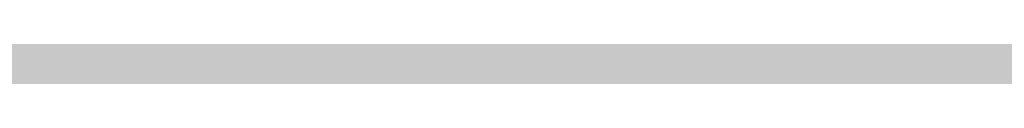
# Model space of a CAD drawing. Units: millimetres. Extents: x 0 to 2267, y 0 to 1823.
# Tile 99 of 256: x 1600.369 to 1605.705, y 1227.331 to 1227.466. Entities that reach past the tile are written whole.
import ezdxf

# ---------------------------------------------------------------- set-up
doc = ezdxf.new("R2010")
doc.units = ezdxf.units.MM
doc.header["$MEASUREMENT"] = 0
doc.layers.add('M-DIMS', color=2, linetype='Continuous', lineweight=25)
doc.layers.add('M-HATC', color=252, linetype='Continuous', lineweight=18)
doc.styles.get("Standard").update_dxf_attribs({"font": 'arial.ttf'})
doc.dimstyles.get("Standard").update_dxf_attribs({"dimtxt": 7, "dimasz": 4, "dimexe": 0.18, "dimexo": 0.0625, "dimgap": 0.09, "dimtad": 0, "dimdec": 0, "dimzin": 0, "dimdsep": 46, "dimtxsty": 'Standard', "dimcen": 0.09, "dimadec": 0, "dimazin": 0, "dimtfac": 1, "dimtdec": 0, "dimtofl": 0, "dimtmove": 0, "dimatfit": 3, "dimfxl": 1, "dimtolj": 1, "dimtzin": 0, "dimarcsym": 0})

# ---------------------------------------------------------------- blocks, each defined once
blk = doc.blocks.new('*D19')
at = {"layer": 'Defpoints', "color": 0, "transparency": 16777216}
for p in [(1605.3399, 1483.3044), (1445.5291, 1333.8851)]:
    blk.add_point(p, dxfattribs=at)
at = {"layer": 'M-DIMS', "color": 0, "lineweight": -2, "transparency": 16777216}
for p, q in [((1605.3399, 1483.2144), (1605.3399, 1483.3944)), ((1605.2499, 1483.3044), (1605.4299, 1483.3044)), ((1366.3244, 1259.8306), (1442.6072, 1331.1532))]:
    blk.add_line(p, q, dxfattribs=at)
at = {"layer": 'M-DIMS', "color": 0, "transparency": 16777216}
blk.add_solid([(1442.1519, 1331.6402), (1443.0625, 1330.6663), (1445.5291, 1333.8851)], dxfattribs=at)
at = {"layer": 'M-DIMS', "color": 0, "transparency": 16777216, "insert": (1349.6425, 1244.2335), "char_height": 7, "attachment_point": 5, "rotation": 43.0753}
blk.add_mtext('\\A1;2X R218.8', dxfattribs=at)

msp = doc.modelspace()

# ---------------------------------------------------------------- hatches: boundary and pattern name
at = {"layer": 'M-HATC'}
h = msp.add_hatch(color=256, dxfattribs=at)
h.dxf.hatch_style = 1
h.paths.add_polyline_path([(2055.771, 1603.062), (1381.0868, 1603.062), (1381.0868, 1598.062), (2055.771, 1598.062)])
h.paths.add_polyline_path([(2055.771, 1598.062), (1381.0868, 1598.062), (1381.0868, 1593.062), (2055.771, 1593.062)])
h.paths.add_polyline_path([(2051.3074, 1536.7609), (1385.5504, 1536.7609), (1385.5504, 1526.7609), (1387.5504, 1526.7609), (1388.5366, 1525.0528), (1385.3319, 1521.2335), (1385.3319, 1521.2226), (2050.2542, 1522.7491), (2048.3212, 1525.0528), (2049.3074, 1526.7609), (2051.3074, 1526.7609)])
edge = h.paths.add_edge_path()
edge.add_arc((1847.5345, 1379.1492), 135, 222.603061, 222.890851, ccw=False)
edge.add_line((1748.1663, 1287.7656), (1683.0921, 1287.7656))
edge.add_arc((1583.7239, 1379.1492), 135, 317.109149, 317.396939, ccw=False)
edge.add_arc((1678.9686, 1290.6707), 5, 222.8909, 317.1091, ccw=False)
edge.add_arc((1774.2133, 1379.1492), 135, 222.603061, 222.890851, ccw=False)
edge.add_line((1674.8451, 1287.7656), (1609.7709, 1287.7656))
edge.add_arc((1510.4027, 1379.1492), 135, 317.109149, 317.396939, ccw=False)
edge.add_arc((1605.6474, 1290.6707), 5, 222.8909, 317.1091, ccw=False)
edge.add_arc((1700.8921, 1379.1492), 135, 222.603061, 222.890851, ccw=False)
edge.add_line((1601.5239, 1287.7656), (1536.4497, 1287.7656))
edge.add_arc((1437.0815, 1379.1492), 135, 317.109149, 317.396939, ccw=False)
edge.add_arc((1532.3262, 1290.6707), 5, 222.8909, 317.1091, ccw=False)
edge.add_arc((1627.5709, 1379.1492), 135, 222.603061, 222.890851, ccw=False)
edge.add_line((1528.2027, 1287.7656), (1505.9289, 1287.7656))
edge.add_spline(control_points=[(1505.9289, 1287.7656), (1504.2622, 1287.7656), (1504.2622, 1282.7656), (1505.9289, 1282.7656)], knot_values=[0, 0, 0, 0, 5, 5, 5, 5], degree=3, periodic=0)
edge.add_line((1505.9289, 1282.7656), (1930.9289, 1282.7656))
edge.add_spline(control_points=[(1930.9289, 1282.7656), (1932.5956, 1282.7656), (1932.5956, 1287.7656), (1930.9289, 1287.7656)], knot_values=[0, 0, 0, 0, 5, 5, 5, 5], degree=3, periodic=0)
edge.add_line((1930.9289, 1287.7656), (1903.0557, 1287.7656))
edge.add_arc((1803.6875, 1379.1492), 135, 317.109149, 317.396939, ccw=False)
edge.add_arc((1898.9322, 1290.6707), 5, 222.8909, 317.1091, ccw=False)
edge.add_arc((1994.1769, 1379.1492), 135, 222.603061, 222.890851, ccw=False)
edge.add_line((1894.8087, 1287.7656), (1829.7345, 1287.7656))
edge.add_arc((1730.3663, 1379.1492), 135, 317.109149, 317.396939, ccw=False)
edge.add_arc((1825.611, 1290.6707), 5, 222.8909, 317.1091, ccw=False)
edge.add_arc((1920.8557, 1379.1492), 135, 222.603061, 222.890851, ccw=False)
edge.add_line((1821.4875, 1287.7656), (1756.4133, 1287.7656))
edge.add_arc((1657.0451, 1379.1492), 135, 317.109149, 317.396939, ccw=False)
edge.add_arc((1752.2898, 1290.6707), 5, 222.8909, 317.1091, ccw=False)
edge = h.paths.add_edge_path()
edge.add_spline(control_points=[(1843.4289, 1227.2475), (1845.0956, 1227.2475), (1845.0956, 1232.2475), (1843.4289, 1232.2475)], knot_values=[0, 0, 0, 0, 5, 5, 5, 5], degree=3, periodic=0)
edge.add_line((1843.4289, 1232.2475), (1593.4289, 1232.2475))
edge.add_spline(control_points=[(1593.4289, 1232.2475), (1591.7622, 1232.2475), (1591.7622, 1227.2475), (1593.4289, 1227.2475)], knot_values=[0, 0, 0, 0, 5, 5, 5, 5], degree=3, periodic=0)
edge.add_line((1593.4289, 1227.2475), (1843.4289, 1227.2475))
h.paths.add_polyline_path([(1905.9289, 1127.4171), (1530.9289, 1127.4171, 0.414214), (1520.9289, 1117.4171), (1530.9289, 1117.4171), (1915.9289, 1117.4171, 0.414214)])
edge = h.paths.add_edge_path()
edge.add_arc((1397.0858, 1498.4078), 12.7299, 90.78215, 190.87871, ccw=False)
edge.add_line((1396.912, 1511.1365), (1428.0097, 1511.3488))
edge.add_line((1428.0097, 1511.3488), (1433.0097, 1511.3488))
edge.add_line((1433.0097, 1511.3488), (1434.439, 1511.3488))
edge.add_arc((1419.474, 1498.0804), 20, 41.561, 74.08211)
edge.add_line((1424.9592, 1517.3135), (1399.9351, 1517.2561))
edge.add_spline(control_points=[(1399.9307, 1517.2561), (1399.884, 1517.2131), (1399.8328, 1517.1689), (1399.7774, 1517.1236)], knot_values=[11.567499, 11.567499, 11.567499, 11.567499, 11.814249, 11.814249, 11.814249, 11.814249], degree=3, periodic=0)
edge.add_spline(control_points=[(1399.6328, 1517.0099), (1399.5831, 1516.9721), (1399.5307, 1516.9338), (1399.4759, 1516.8947)], knot_values=[11.167718, 11.167718, 11.167718, 11.167718, 11.365188, 11.365188, 11.365188, 11.365188], degree=3, periodic=0)
edge.add_spline(control_points=[(1399.3398, 1516.8001), (1399.1514, 1516.6719), (1398.9384, 1516.5377), (1398.704, 1516.3994)], knot_values=[10.376405, 10.376405, 10.376405, 10.376405, 11.00994, 11.00994, 11.00994, 11.00994], degree=3, periodic=0)
edge.add_spline(control_points=[(1398.6572, 1516.3719), (1398.5789, 1516.326), (1398.4983, 1516.2797), (1398.4155, 1516.2331)], knot_values=[10.125175, 10.125175, 10.125175, 10.125175, 10.334406, 10.334406, 10.334406, 10.334406], degree=3, periodic=0)
edge.add_spline(control_points=[(1398.2642, 1516.1487), (1398.196, 1516.1111), (1398.1263, 1516.0732), (1398.0555, 1516.0351)], knot_values=[9.832246, 9.832246, 9.832246, 9.832246, 9.999658, 9.999658, 9.999658, 9.999658], degree=3, periodic=0)
edge.add_spline(control_points=[(1397.9987, 1516.0048), (1397.7312, 1515.8621), (1397.446, 1515.7171), (1397.1466, 1515.5714)], knot_values=[9.161808, 9.161808, 9.161808, 9.161808, 9.787769, 9.787769, 9.787769, 9.787769], degree=3, periodic=0)
edge.add_spline(control_points=[(1397.1466, 1515.5714), (1396.8418, 1515.423), (1396.5222, 1515.274), (1396.1914, 1515.1262)], knot_values=[8.524455, 8.524455, 8.524455, 8.524455, 9.161808, 9.161808, 9.161808, 9.161808], degree=3, periodic=0)
edge.add_spline(control_points=[(1396.0777, 1515.0756), (1395.9854, 1515.0348), (1395.8922, 1514.994), (1395.7983, 1514.9534)], knot_values=[8.275193, 8.275193, 8.275193, 8.275193, 8.451726, 8.451726, 8.451726, 8.451726], degree=3, periodic=0)
edge.add_spline(control_points=[(1395.6018, 1514.8691), (1395.4997, 1514.8257), (1395.3968, 1514.7824), (1395.2932, 1514.7394)], knot_values=[7.962917, 7.962917, 7.962917, 7.962917, 8.152764, 8.152764, 8.152764, 8.152764], degree=3, periodic=0)
edge.add_spline(control_points=[(1395.2116, 1514.7057), (1394.8278, 1514.5475), (1394.4345, 1514.3929), (1394.0364, 1514.2442)], knot_values=[7.21254, 7.21254, 7.21254, 7.21254, 7.913148, 7.913148, 7.913148, 7.913148], degree=3, periodic=0)
edge.add_spline(control_points=[(1394.0364, 1514.2442), (1393.7076, 1514.1214), (1393.3754, 1514.0027), (1393.0427, 1513.8895)], knot_values=[6.633733, 6.633733, 6.633733, 6.633733, 7.21254, 7.21254, 7.21254, 7.21254], degree=3, periodic=0)
edge.add_spline(control_points=[(1392.8214, 1513.815), (1392.7198, 1513.7812), (1392.6181, 1513.7479), (1392.5166, 1513.7152)], knot_values=[6.328796, 6.328796, 6.328796, 6.328796, 6.505493, 6.505493, 6.505493, 6.505493], degree=3, periodic=0)
edge.add_spline(control_points=[(1392.5166, 1513.7152), (1392.3187, 1513.6515), (1392.1212, 1513.59), (1391.9244, 1513.531)], knot_values=[5.984605, 5.984605, 5.984605, 5.984605, 6.328796, 6.328796, 6.328796, 6.328796], degree=3, periodic=0)
edge.add_spline(control_points=[(1391.7915, 1513.4915), (1391.3122, 1513.3501), (1390.8384, 1513.2239), (1390.3784, 1513.1171)], knot_values=[5.066697, 5.066697, 5.066697, 5.066697, 5.907055, 5.907055, 5.907055, 5.907055], degree=3, periodic=0)
edge.add_spline(control_points=[(1390.3784, 1513.1171), (1390.1797, 1513.071), (1389.9836, 1513.0284), (1389.7907, 1512.9899)], knot_values=[4.70367, 4.70367, 4.70367, 4.70367, 5.066695, 5.066695, 5.066695, 5.066695], degree=3, periodic=0)
edge.add_spline(control_points=[(1389.422, 1512.9204), (1389.2459, 1512.8892), (1389.0729, 1512.8617), (1388.9036, 1512.8381)], knot_values=[4.130571, 4.130571, 4.130571, 4.130571, 4.469816, 4.469816, 4.469816, 4.469816], degree=3, periodic=0)
edge.add_spline(control_points=[(1388.9036, 1512.8381), (1388.591, 1512.7946), (1388.2911, 1512.7644), (1388.0071, 1512.7494)], knot_values=[3.504031, 3.504031, 3.504031, 3.504031, 4.130571, 4.130571, 4.130571, 4.130571], degree=3, periodic=0)
edge.add_spline(control_points=[(1387.9356, 1512.7459), (1387.8538, 1512.7423), (1387.7733, 1512.74), (1387.6944, 1512.739)], knot_values=[3.268866, 3.268866, 3.268866, 3.268866, 3.451164, 3.451164, 3.451164, 3.451164], degree=3, periodic=0)
edge.add_spline(control_points=[(1387.3351, 1512.7443), (1387.2076, 1512.7499), (1387.0847, 1512.7597), (1386.967, 1512.7739)], knot_values=[2.670686, 2.670686, 2.670686, 2.670686, 2.984, 2.984, 2.984, 2.984], degree=3, periodic=0)
edge.add_spline(control_points=[(1386.8327, 1512.7922), (1386.8209, 1512.7941), (1386.8092, 1512.7959), (1386.7975, 1512.7979)], knot_values=[2.516981, 2.516981, 2.516981, 2.516981, 2.549528, 2.549528, 2.549528, 2.549528], degree=3, periodic=0)
edge.add_spline(control_points=[(1386.4526, 1512.8735), (1386.4257, 1512.881), (1386.3993, 1512.889), (1386.3733, 1512.8972)], knot_values=[2.095869, 2.095869, 2.095869, 2.095869, 2.17941, 2.17941, 2.17941, 2.17941], degree=3, periodic=0)
edge.add_spline(control_points=[(1386.0691, 1513.0189), (1386.0634, 1513.0217), (1386.0577, 1513.0246), (1386.052, 1513.0275)], knot_values=[1.72453, 1.72453, 1.72453, 1.72453, 1.745933, 1.745933, 1.745933, 1.745933], degree=3, periodic=0)
edge.add_arc((1399.474, 1498.0804), 20, 131.82432, 180)
edge.add_arc((1630.3336, 1505.5484), 250.9708, 181.705176, 236.427975)
edge.add_arc((1605.3399, 1483.3044), 218.7822, 238.660829, 243.34961)
edge.add_arc((1647.0911, 1510.3592), 262.8986, 183.129836, 237.853442, ccw=False)
h.paths.add_polyline_path([(1406.5369, 1391.9644, 0.149382), (1491.5506, 1296.4418, -0.129517)], flags=17)
edge = h.paths.add_edge_path()
edge.add_arc((2037.3838, 1498.0804), 20, 0, 48.26587)
edge.add_spline(control_points=[(2050.6973, 1513.0052), (2050.6512, 1512.9847), (2050.6034, 1512.9655), (2050.5539, 1512.9477)], knot_values=[1.835652, 1.835652, 1.835652, 1.835652, 2.000781, 2.000781, 2.000781, 2.000781], degree=3, periodic=0)
edge.add_spline(control_points=[(2050.4616, 1512.9166), (2050.479, 1512.9221), (2050.4963, 1512.9277), (2050.5133, 1512.9335)], knot_values=[2.045477, 2.045477, 2.045477, 2.045477, 2.101389, 2.101389, 2.101389, 2.101389], degree=3, periodic=0)
edge.add_spline(control_points=[(2050.129, 1512.8342), (2050.1984, 1512.8473), (2050.2657, 1512.8623), (2050.3308, 1512.8792)], knot_values=[2.237629, 2.237629, 2.237629, 2.237629, 2.435841, 2.435841, 2.435841, 2.435841], degree=3, periodic=0)
edge.add_spline(control_points=[(2050.0946, 1512.8278), (2050.1061, 1512.8299), (2050.1176, 1512.832), (2050.129, 1512.8342)], knot_values=[2.435841, 2.435841, 2.435841, 2.435841, 2.468321, 2.468321, 2.468321, 2.468321], degree=3, periodic=0)
edge.add_spline(control_points=[(2049.7843, 1512.7851), (2049.8552, 1512.7922), (2049.9243, 1512.8008), (2049.9917, 1512.8109)], knot_values=[2.563852, 2.563852, 2.563852, 2.563852, 2.748541, 2.748541, 2.748541, 2.748541], degree=3, periodic=0)
edge.add_spline(control_points=[(2049.4052, 1512.7617), (2049.5364, 1512.7653), (2049.6629, 1512.773), (2049.7843, 1512.7851)], knot_values=[2.748541, 2.748541, 2.748541, 2.748541, 3.064882, 3.064882, 3.064882, 3.064882], degree=3, periodic=0)
edge.add_spline(control_points=[(2049.1698, 1512.7597), (2049.2336, 1512.7591), (2049.2965, 1512.7594), (2049.3584, 1512.7606)], knot_values=[3.102309, 3.102309, 3.102309, 3.102309, 3.2503, 3.2503, 3.2503, 3.2503], degree=3, periodic=0)
edge.add_spline(control_points=[(2048.8573, 1512.7691), (2048.9638, 1512.7638), (2049.068, 1512.7606), (2049.1698, 1512.7597)], knot_values=[3.2503, 3.2503, 3.2503, 3.2503, 3.486069, 3.486069, 3.486069, 3.486069], degree=3, periodic=0)
edge.add_spline(control_points=[(2048.6924, 1512.7789), (2048.3729, 1512.8009), (2048.0345, 1512.8411), (2047.6817, 1512.897)], knot_values=[3.606429, 3.606429, 3.606429, 3.606429, 4.2989, 4.2989, 4.2989, 4.2989], degree=3, periodic=0)
edge.add_spline(control_points=[(2047.6817, 1512.897), (2047.5458, 1512.9185), (2047.4077, 1512.9424), (2047.2678, 1512.9685)], knot_values=[4.2989, 4.2989, 4.2989, 4.2989, 4.565769, 4.565769, 4.565769, 4.565769], degree=3, periodic=0)
edge.add_spline(control_points=[(2047.2678, 1512.9685), (2047.1449, 1512.9914), (2047.0207, 1513.016), (2046.8951, 1513.0422)], knot_values=[4.565769, 4.565769, 4.565769, 4.565769, 4.799971, 4.799971, 4.799971, 4.799971], degree=3, periodic=0)
edge.add_spline(control_points=[(2046.8951, 1513.0422), (2046.5286, 1513.1188), (2046.1513, 1513.209), (2045.7676, 1513.3107)], knot_values=[4.799971, 4.799971, 4.799971, 4.799971, 5.483718, 5.483718, 5.483718, 5.483718], degree=3, periodic=0)
edge.add_spline(control_points=[(2045.7676, 1513.3107), (2045.3724, 1513.4154), (2044.9704, 1513.5322), (2044.5662, 1513.6588)], knot_values=[5.483718, 5.483718, 5.483718, 5.483718, 6.187866, 6.187866, 6.187866, 6.187866], degree=3, periodic=0)
edge.add_spline(control_points=[(2044.5662, 1513.6588), (2044.4149, 1513.7061), (2044.2633, 1513.7549), (2044.1116, 1513.8048)], knot_values=[6.187866, 6.187866, 6.187866, 6.187866, 6.451551, 6.451551, 6.451551, 6.451551], degree=3, periodic=0)
edge.add_spline(control_points=[(2044.1116, 1513.8048), (2043.9967, 1513.8427), (2043.8817, 1513.8813), (2043.7668, 1513.9205)], knot_values=[6.451551, 6.451551, 6.451551, 6.451551, 6.651434, 6.651434, 6.651434, 6.651434], degree=3, periodic=0)
edge.add_spline(control_points=[(2043.7668, 1513.9205), (2043.3716, 1514.0554), (2042.9774, 1514.1979), (2042.5886, 1514.3458)], knot_values=[6.651434, 6.651434, 6.651434, 6.651434, 7.338879, 7.338879, 7.338879, 7.338879], degree=3, periodic=0)
edge.add_spline(control_points=[(2042.5886, 1514.3458), (2042.1643, 1514.5071), (2041.7465, 1514.6749), (2041.3409, 1514.846)], knot_values=[7.338879, 7.338879, 7.338879, 7.338879, 8.089209, 8.089209, 8.089209, 8.089209], degree=3, periodic=0)
edge.add_spline(control_points=[(2041.3409, 1514.846), (2041.1028, 1514.9465), (2040.869, 1515.0481), (2040.6405, 1515.1502)], knot_values=[8.089209, 8.089209, 8.089209, 8.089209, 8.529587, 8.529587, 8.529587, 8.529587], degree=3, periodic=0)
edge.add_spline(control_points=[(2040.51, 1515.2089), (2040.0824, 1515.4022), (2039.6747, 1515.5971), (2039.295, 1515.7894)], knot_values=[8.613818, 8.613818, 8.613818, 8.613818, 9.44571, 9.44571, 9.44571, 9.44571], degree=3, periodic=0)
edge.add_spline(control_points=[(2039.295, 1515.7894), (2039.0618, 1515.9075), (2038.8391, 1516.0246), (2038.6288, 1516.1398)], knot_values=[9.44571, 9.44571, 9.44571, 9.44571, 9.956404, 9.956404, 9.956404, 9.956404], degree=3, periodic=0)
edge.add_spline(control_points=[(2038.6288, 1516.1398), (2038.5187, 1516.2001), (2038.4121, 1516.2598), (2038.309, 1516.3189)], knot_values=[9.956404, 9.956404, 9.956404, 9.956404, 10.223542, 10.223542, 10.223542, 10.223542], degree=3, periodic=0)
edge.add_spline(control_points=[(2038.309, 1516.3189), (2038.2138, 1516.3735), (2038.1216, 1516.4276), (2038.0328, 1516.481)], knot_values=[10.223542, 10.223542, 10.223542, 10.223542, 10.47051, 10.47051, 10.47051, 10.47051], degree=3, periodic=0)
edge.add_spline(control_points=[(2038.0328, 1516.481), (2037.7855, 1516.6296), (2037.5639, 1516.773), (2037.3722, 1516.909)], knot_values=[10.47051, 10.47051, 10.47051, 10.47051, 11.15767, 11.15767, 11.15767, 11.15767], degree=3, periodic=0)
edge.add_spline(control_points=[(2037.3722, 1516.909), (2037.2789, 1516.9752), (2037.1927, 1517.0396), (2037.1142, 1517.102)], knot_values=[11.15767, 11.15767, 11.15767, 11.15767, 11.49227, 11.49227, 11.49227, 11.49227], degree=3, periodic=0)
edge.add_spline(control_points=[(2036.8564, 1517.3259), (2036.9148, 1517.2692), (2036.9814, 1517.2103), (2037.0557, 1517.1492)], knot_values=[11.577341, 11.577341, 11.577341, 11.577341, 11.91035, 11.91035, 11.91035, 11.91035], degree=3, periodic=0)
edge.add_spline(control_points=[(2036.8074, 1517.3748), (2036.823, 1517.3587), (2036.8393, 1517.3424), (2036.8564, 1517.3259)], knot_values=[11.91035, 11.91035, 11.91035, 11.91035, 12.007402, 12.007402, 12.007402, 12.007402], degree=3, periodic=0)
edge.add_spline(control_points=[(2036.7017, 1517.494), (2036.7104, 1517.483), (2036.7196, 1517.4719), (2036.7291, 1517.4606)], knot_values=[12.184155, 12.184155, 12.184155, 12.184155, 12.255409, 12.255409, 12.255409, 12.255409], degree=3, periodic=0)
edge.add_spline(control_points=[(2036.6159, 1517.6205), (2036.62, 1517.613), (2036.6243, 1517.6055), (2036.6289, 1517.5979)], knot_values=[12.487913, 12.487913, 12.487913, 12.487913, 12.541035, 12.541035, 12.541035, 12.541035], degree=3, periodic=0)
edge.add_spline(control_points=[(2036.5635, 1517.786), (2036.5637, 1517.7794), (2036.5642, 1517.7726), (2036.565, 1517.7658)], knot_values=[12.911761, 12.911761, 12.911761, 12.911761, 12.968286, 12.968286, 12.968286, 12.968286], degree=3, periodic=0)
edge.add_spline(control_points=[(2036.6166, 1517.9304), (2036.6125, 1517.9259), (2036.6086, 1517.9212), (2036.6049, 1517.9165)], knot_values=[13.382527, 13.382527, 13.382527, 13.382527, 13.433791, 13.433791, 13.433791, 13.433791], degree=3, periodic=0)
edge.add_spline(control_points=[(2036.749, 1518.017), (2036.7361, 1518.0116), (2036.7239, 1518.006), (2036.7124, 1518.0002)], knot_values=[13.726299, 13.726299, 13.726299, 13.726299, 13.809928, 13.809928, 13.809928, 13.809928], degree=3, periodic=0)
edge.add_spline(control_points=[(2036.8604, 1518.0528), (2036.8386, 1518.0474), (2036.8181, 1518.0416), (2036.7988, 1518.0353)], knot_values=[13.910887, 13.910887, 13.910887, 13.910887, 14.02153, 14.02153, 14.02153, 14.02153], degree=3, periodic=0)
edge.add_line((2036.9639, 1518.0804), (2032.3838, 1518.0804))
edge.add_line((2032.3838, 1518.0804), (2027.3838, 1518.0804))
edge.add_line((2027.3838, 1518.0804), (2022.3838, 1518.0804))
edge.add_line((2022.3838, 1518.0804), (2017.3838, 1518.0804))
edge.add_arc((2017.3838, 1498.0804), 20, 90, 138.439)
edge.add_line((2002.4188, 1511.3488), (2003.8481, 1511.3488))
edge.add_line((2003.8481, 1511.3488), (2008.8481, 1511.3488))
edge.add_line((2008.8481, 1511.3488), (2039.772, 1511.1377))
edge.add_arc((2039.772, 1498.4078), 12.7299, -10.87871, 90, ccw=False)
edge.add_arc((1789.7668, 1510.3592), 262.8986, 302.146558, 356.870164, ccw=False)
edge.add_arc((1831.5179, 1483.3044), 218.7822, 296.65039, 301.339171)
edge.add_arc((1806.5242, 1505.5484), 250.9708, 303.572025, 358.294824)
h.paths.add_polyline_path([(2030.321, 1391.9644, -0.129517), (1945.3072, 1296.4418, 0.149382)], flags=17)
edge = h.paths.add_edge_path()
edge.add_spline(control_points=[(2037.2464, 1518.0821), (2037.2898, 1518.081), (2037.3355, 1518.0804), (2037.3838, 1518.0804)], knot_values=[0.000012, 0.000012, 0.000012, 0.000012, 0.144754, 0.144754, 0.144754, 0.144754], degree=3, periodic=0)
edge.add_line((2037.3357, 1518.0804), (2037.0096, 1518.0804))
edge.add_spline(control_points=[(2037.0096, 1518.0804), (2036.9822, 1518.0768), (2036.956, 1518.0727), (2036.9312, 1518.0681)], knot_values=[14.13465, 14.13465, 14.13465, 14.13465, 14.247197, 14.247197, 14.247197, 14.247197], degree=3, periodic=0)
edge.add_spline(control_points=[(2036.9312, 1518.0681), (2036.9276, 1518.0674), (2036.9241, 1518.0667), (2036.9205, 1518.0661)], knot_values=[14.118315, 14.118315, 14.118315, 14.118315, 14.13465, 14.13465, 14.13465, 14.13465], degree=3, periodic=0)
edge.add_spline(control_points=[(2036.9205, 1518.0661), (2036.9118, 1518.0644), (2036.9032, 1518.0626), (2036.8948, 1518.0608)], knot_values=[14.078086, 14.078086, 14.078086, 14.078086, 14.118315, 14.118315, 14.118315, 14.118315], degree=3, periodic=0)
edge.add_spline(control_points=[(2036.8948, 1518.0608), (2036.883, 1518.0583), (2036.8716, 1518.0556), (2036.8604, 1518.0528)], knot_values=[14.02153, 14.02153, 14.02153, 14.02153, 14.078086, 14.078086, 14.078086, 14.078086], degree=3, periodic=0)
edge.add_spline(control_points=[(2036.8604, 1518.0528), (2036.8386, 1518.0474), (2036.8181, 1518.0416), (2036.7988, 1518.0353)], knot_values=[13.910887, 13.910887, 13.910887, 13.910887, 14.02153, 14.02153, 14.02153, 14.02153], degree=3, periodic=0)
edge.add_spline(control_points=[(2036.7988, 1518.0353), (2036.7981, 1518.035), (2036.7974, 1518.0348), (2036.7967, 1518.0346)], knot_values=[13.906906, 13.906906, 13.906906, 13.906906, 13.910887, 13.910887, 13.910887, 13.910887], degree=3, periodic=0)
edge.add_spline(control_points=[(2036.7967, 1518.0346), (2036.7882, 1518.0318), (2036.7799, 1518.0289), (2036.7719, 1518.0259)], knot_values=[13.857826, 13.857826, 13.857826, 13.857826, 13.906906, 13.906906, 13.906906, 13.906906], degree=3, periodic=0)
edge.add_spline(control_points=[(2036.7719, 1518.0259), (2036.764, 1518.023), (2036.7564, 1518.02), (2036.749, 1518.017)], knot_values=[13.809928, 13.809928, 13.809928, 13.809928, 13.857826, 13.857826, 13.857826, 13.857826], degree=3, periodic=0)
edge.add_spline(control_points=[(2036.749, 1518.017), (2036.7361, 1518.0116), (2036.7239, 1518.006), (2036.7124, 1518.0002)], knot_values=[13.726299, 13.726299, 13.726299, 13.726299, 13.809928, 13.809928, 13.809928, 13.809928], degree=3, periodic=0)
edge.add_spline(control_points=[(2036.7124, 1518.0002), (2036.7121, 1518), (2036.7118, 1517.9999), (2036.7115, 1517.9997)], knot_values=[13.723993, 13.723993, 13.723993, 13.723993, 13.726299, 13.726299, 13.726299, 13.726299], degree=3, periodic=0)
edge.add_spline(control_points=[(2036.7115, 1517.9997), (2036.7063, 1517.9971), (2036.7013, 1517.9944), (2036.6965, 1517.9917)], knot_values=[13.686536, 13.686536, 13.686536, 13.686536, 13.723993, 13.723993, 13.723993, 13.723993], degree=3, periodic=0)
edge.add_spline(control_points=[(2036.6965, 1517.9917), (2036.6919, 1517.9891), (2036.6874, 1517.9865), (2036.6831, 1517.9839)], knot_values=[13.651251, 13.651251, 13.651251, 13.651251, 13.686536, 13.686536, 13.686536, 13.686536], degree=3, periodic=0)
edge.add_spline(control_points=[(2036.6831, 1517.9839), (2036.6764, 1517.9798), (2036.67, 1517.9757), (2036.6639, 1517.9714)], knot_values=[13.596804, 13.596804, 13.596804, 13.596804, 13.651251, 13.651251, 13.651251, 13.651251], degree=3, periodic=0)
edge.add_spline(control_points=[(2036.6639, 1517.9714), (2036.6636, 1517.9712), (2036.6633, 1517.9709), (2036.6629, 1517.9707)], knot_values=[13.593956, 13.593956, 13.593956, 13.593956, 13.596804, 13.596804, 13.596804, 13.596804], degree=3, periodic=0)
edge.add_spline(control_points=[(2036.6629, 1517.9707), (2036.6603, 1517.9689), (2036.6577, 1517.967), (2036.6552, 1517.9651)], knot_values=[13.570322, 13.570322, 13.570322, 13.570322, 13.593956, 13.593956, 13.593956, 13.593956], degree=3, periodic=0)
edge.add_spline(control_points=[(2036.6552, 1517.9651), (2036.6525, 1517.9631), (2036.6499, 1517.9611), (2036.6474, 1517.9591)], knot_values=[13.545477, 13.545477, 13.545477, 13.545477, 13.570322, 13.570322, 13.570322, 13.570322], degree=3, periodic=0)
edge.add_spline(control_points=[(2036.6474, 1517.9591), (2036.6472, 1517.9589), (2036.6471, 1517.9588), (2036.6469, 1517.9587)], knot_values=[13.543931, 13.543931, 13.543931, 13.543931, 13.545477, 13.545477, 13.545477, 13.545477], degree=3, periodic=0)
edge.add_spline(control_points=[(2036.6469, 1517.9587), (2036.6412, 1517.9541), (2036.6358, 1517.9494), (2036.6307, 1517.9447)], knot_values=[13.488237, 13.488237, 13.488237, 13.488237, 13.543931, 13.543931, 13.543931, 13.543931], degree=3, periodic=0)
edge.add_spline(control_points=[(2036.6307, 1517.9447), (2036.6282, 1517.9423), (2036.6257, 1517.9399), (2036.6233, 1517.9374)], knot_values=[13.460307, 13.460307, 13.460307, 13.460307, 13.488237, 13.488237, 13.488237, 13.488237], degree=3, periodic=0)
edge.add_spline(control_points=[(2036.6233, 1517.9374), (2036.6215, 1517.9356), (2036.6198, 1517.9338), (2036.6181, 1517.932)], knot_values=[13.439712, 13.439712, 13.439712, 13.439712, 13.460307, 13.460307, 13.460307, 13.460307], degree=3, periodic=0)
edge.add_spline(control_points=[(2036.6181, 1517.932), (2036.6176, 1517.9315), (2036.6171, 1517.9309), (2036.6166, 1517.9304)], knot_values=[13.433791, 13.433791, 13.433791, 13.433791, 13.439712, 13.439712, 13.439712, 13.439712], degree=3, periodic=0)
edge.add_spline(control_points=[(2036.6166, 1517.9304), (2036.6125, 1517.9259), (2036.6086, 1517.9212), (2036.6049, 1517.9165)], knot_values=[13.382527, 13.382527, 13.382527, 13.382527, 13.433791, 13.433791, 13.433791, 13.433791], degree=3, periodic=0)
edge.add_spline(control_points=[(2036.6049, 1517.9165), (2036.6026, 1517.9135), (2036.6004, 1517.9104), (2036.5982, 1517.9074)], knot_values=[13.350017, 13.350017, 13.350017, 13.350017, 13.382527, 13.382527, 13.382527, 13.382527], degree=3, periodic=0)
edge.add_spline(control_points=[(2036.5982, 1517.9074), (2036.5972, 1517.9059), (2036.5962, 1517.9043), (2036.5952, 1517.9028)], knot_values=[13.333922, 13.333922, 13.333922, 13.333922, 13.350017, 13.350017, 13.350017, 13.350017], degree=3, periodic=0)
edge.add_spline(control_points=[(2036.5952, 1517.9028), (2036.5945, 1517.9018), (2036.5939, 1517.9009), (2036.5933, 1517.8999)], knot_values=[13.323828, 13.323828, 13.323828, 13.323828, 13.333922, 13.333922, 13.333922, 13.333922], degree=3, periodic=0)
edge.add_spline(control_points=[(2036.5933, 1517.8999), (2036.5905, 1517.8955), (2036.5879, 1517.8909), (2036.5855, 1517.8864)], knot_values=[13.277545, 13.277545, 13.277545, 13.277545, 13.323828, 13.323828, 13.323828, 13.323828], degree=3, periodic=0)
edge.add_spline(control_points=[(2036.5855, 1517.8864), (2036.5836, 1517.8827), (2036.5817, 1517.8789), (2036.5801, 1517.8751)], knot_values=[13.240119, 13.240119, 13.240119, 13.240119, 13.277545, 13.277545, 13.277545, 13.277545], degree=3, periodic=0)
edge.add_spline(control_points=[(2036.5801, 1517.8751), (2036.5795, 1517.8739), (2036.579, 1517.8727), (2036.5785, 1517.8715)], knot_values=[13.228211, 13.228211, 13.228211, 13.228211, 13.240119, 13.240119, 13.240119, 13.240119], degree=3, periodic=0)
edge.add_spline(control_points=[(2036.5785, 1517.8715), (2036.578, 1517.8702), (2036.5774, 1517.869), (2036.5769, 1517.8677)], knot_values=[13.215717, 13.215717, 13.215717, 13.215717, 13.228211, 13.228211, 13.228211, 13.228211], degree=3, periodic=0)
edge.add_spline(control_points=[(2036.5769, 1517.8677), (2036.5755, 1517.864), (2036.5741, 1517.8603), (2036.5729, 1517.8565)], knot_values=[13.179847, 13.179847, 13.179847, 13.179847, 13.215717, 13.215717, 13.215717, 13.215717], degree=3, periodic=0)
edge.add_spline(control_points=[(2036.5729, 1517.8565), (2036.5713, 1517.8515), (2036.5699, 1517.8464), (2036.5687, 1517.8413)], knot_values=[13.132017, 13.132017, 13.132017, 13.132017, 13.179847, 13.179847, 13.179847, 13.179847], degree=3, periodic=0)
edge.add_spline(control_points=[(2036.5687, 1517.8413), (2036.5684, 1517.8402), (2036.5682, 1517.8392), (2036.568, 1517.8382)], knot_values=[13.122482, 13.122482, 13.122482, 13.122482, 13.132017, 13.132017, 13.132017, 13.132017], degree=3, periodic=0)
edge.add_spline(control_points=[(2036.568, 1517.8382), (2036.5676, 1517.8363), (2036.5672, 1517.8345), (2036.5669, 1517.8327)], knot_values=[13.105592, 13.105592, 13.105592, 13.105592, 13.122482, 13.122482, 13.122482, 13.122482], degree=3, periodic=0)
edge.add_spline(control_points=[(2036.5669, 1517.8327), (2036.5662, 1517.8292), (2036.5657, 1517.8257), (2036.5652, 1517.8222)], knot_values=[13.074063, 13.074063, 13.074063, 13.074063, 13.105592, 13.105592, 13.105592, 13.105592], degree=3, periodic=0)
edge.add_spline(control_points=[(2036.5652, 1517.8222), (2036.5652, 1517.8222), (2036.5652, 1517.8222), (2036.5652, 1517.8222)], knot_values=[13.074043, 13.074043, 13.074043, 13.074043, 13.074063, 13.074063, 13.074063, 13.074063], degree=3, periodic=0)
edge.add_spline(control_points=[(2036.5652, 1517.8222), (2036.5644, 1517.8164), (2036.5639, 1517.8106), (2036.5636, 1517.8046)], knot_values=[13.021884, 13.021884, 13.021884, 13.021884, 13.074043, 13.074043, 13.074043, 13.074043], degree=3, periodic=0)
edge.add_spline(control_points=[(2036.5636, 1517.8046), (2036.5636, 1517.804), (2036.5636, 1517.8034), (2036.5635, 1517.8028)], knot_values=[13.01674, 13.01674, 13.01674, 13.01674, 13.021884, 13.021884, 13.021884, 13.021884], degree=3, periodic=0)
edge.add_spline(control_points=[(2036.5635, 1517.8028), (2036.5634, 1517.8005), (2036.5634, 1517.7982), (2036.5634, 1517.7958)], knot_values=[12.996438, 12.996438, 12.996438, 12.996438, 13.01674, 13.01674, 13.01674, 13.01674], degree=3, periodic=0)
edge.add_spline(control_points=[(2036.5634, 1517.7958), (2036.5633, 1517.7926), (2036.5634, 1517.7893), (2036.5635, 1517.786)], knot_values=[12.968286, 12.968286, 12.968286, 12.968286, 12.996438, 12.996438, 12.996438, 12.996438], degree=3, periodic=0)
edge.add_spline(control_points=[(2036.5635, 1517.786), (2036.5637, 1517.7794), (2036.5642, 1517.7726), (2036.565, 1517.7658)], knot_values=[12.911761, 12.911761, 12.911761, 12.911761, 12.968286, 12.968286, 12.968286, 12.968286], degree=3, periodic=0)
edge.add_spline(control_points=[(2036.565, 1517.7658), (2036.565, 1517.7657), (2036.565, 1517.7656), (2036.565, 1517.7656)], knot_values=[12.911017, 12.911017, 12.911017, 12.911017, 12.911761, 12.911761, 12.911761, 12.911761], degree=3, periodic=0)
edge.add_spline(control_points=[(2036.565, 1517.7656), (2036.5654, 1517.7625), (2036.5658, 1517.7593), (2036.5663, 1517.7562)], knot_values=[12.88528, 12.88528, 12.88528, 12.88528, 12.911017, 12.911017, 12.911017, 12.911017], degree=3, periodic=0)
edge.add_spline(control_points=[(2036.5663, 1517.7562), (2036.5667, 1517.7534), (2036.5672, 1517.7506), (2036.5677, 1517.7478)], knot_values=[12.862519, 12.862519, 12.862519, 12.862519, 12.88528, 12.88528, 12.88528, 12.88528], degree=3, periodic=0)
edge.add_spline(control_points=[(2036.5677, 1517.7478), (2036.5678, 1517.7474), (2036.5679, 1517.7469), (2036.568, 1517.7465)], knot_values=[12.858885, 12.858885, 12.858885, 12.858885, 12.862519, 12.862519, 12.862519, 12.862519], degree=3, periodic=0)
edge.add_spline(control_points=[(2036.568, 1517.7465), (2036.5692, 1517.7399), (2036.5707, 1517.7332), (2036.5724, 1517.7264)], knot_values=[12.8053, 12.8053, 12.8053, 12.8053, 12.858885, 12.858885, 12.858885, 12.858885], degree=3, periodic=0)
edge.add_spline(control_points=[(2036.5724, 1517.7264), (2036.5734, 1517.7226), (2036.5745, 1517.7187), (2036.5756, 1517.7149)], knot_values=[12.775176, 12.775176, 12.775176, 12.775176, 12.8053, 12.8053, 12.8053, 12.8053], degree=3, periodic=0)
edge.add_spline(control_points=[(2036.5756, 1517.7149), (2036.5763, 1517.7125), (2036.577, 1517.7102), (2036.5778, 1517.7078)], knot_values=[12.756759, 12.756759, 12.756759, 12.756759, 12.775176, 12.775176, 12.775176, 12.775176], degree=3, periodic=0)
edge.add_spline(control_points=[(2036.5778, 1517.7078), (2036.5781, 1517.7067), (2036.5784, 1517.7057), (2036.5787, 1517.7047)], knot_values=[12.748742, 12.748742, 12.748742, 12.748742, 12.756759, 12.756759, 12.756759, 12.756759], degree=3, periodic=0)
edge.add_spline(control_points=[(2036.5787, 1517.7047), (2036.5808, 1517.6983), (2036.5831, 1517.6919), (2036.5856, 1517.6854)], knot_values=[12.69959, 12.69959, 12.69959, 12.69959, 12.748742, 12.748742, 12.748742, 12.748742], degree=3, periodic=0)
edge.add_spline(control_points=[(2036.5856, 1517.6854), (2036.5876, 1517.68), (2036.5898, 1517.6746), (2036.5921, 1517.6692)], knot_values=[12.659038, 12.659038, 12.659038, 12.659038, 12.69959, 12.69959, 12.69959, 12.69959], degree=3, periodic=0)
edge.add_spline(control_points=[(2036.5921, 1517.6692), (2036.594, 1517.6648), (2036.5959, 1517.6605), (2036.5979, 1517.6561)], knot_values=[12.626806, 12.626806, 12.626806, 12.626806, 12.659038, 12.659038, 12.659038, 12.659038], degree=3, periodic=0)
edge.add_spline(control_points=[(2036.5979, 1517.6561), (2036.5984, 1517.6551), (2036.5989, 1517.6541), (2036.5993, 1517.6531)], knot_values=[12.619394, 12.619394, 12.619394, 12.619394, 12.626806, 12.626806, 12.626806, 12.626806], degree=3, periodic=0)
edge.add_spline(control_points=[(2036.5993, 1517.6531), (2036.6043, 1517.6424), (2036.6099, 1517.6315), (2036.6159, 1517.6205)], knot_values=[12.541039, 12.541039, 12.541039, 12.541039, 12.619394, 12.619394, 12.619394, 12.619394], degree=3, periodic=0)
edge.add_spline(control_points=[(2036.6159, 1517.6205), (2036.6159, 1517.6205), (2036.6159, 1517.6205), (2036.6159, 1517.6205)], knot_values=[12.541035, 12.541035, 12.541035, 12.541035, 12.541039, 12.541039, 12.541039, 12.541039], degree=3, periodic=0)
edge.add_spline(control_points=[(2036.6159, 1517.6205), (2036.62, 1517.613), (2036.6243, 1517.6055), (2036.6289, 1517.5979)], knot_values=[12.487913, 12.487913, 12.487913, 12.487913, 12.541035, 12.541035, 12.541035, 12.541035], degree=3, periodic=0)
edge.add_spline(control_points=[(2036.6289, 1517.5979), (2036.6326, 1517.5916), (2036.6365, 1517.5853), (2036.6406, 1517.5789)], knot_values=[12.443982, 12.443982, 12.443982, 12.443982, 12.487913, 12.487913, 12.487913, 12.487913], degree=3, periodic=0)
edge.add_spline(control_points=[(2036.6406, 1517.5789), (2036.6414, 1517.5776), (2036.6423, 1517.5763), (2036.6431, 1517.5749)], knot_values=[12.434996, 12.434996, 12.434996, 12.434996, 12.443982, 12.443982, 12.443982, 12.443982], degree=3, periodic=0)
edge.add_spline(control_points=[(2036.6431, 1517.5749), (2036.6531, 1517.5596), (2036.6639, 1517.5439), (2036.6756, 1517.528)], knot_values=[12.329647, 12.329647, 12.329647, 12.329647, 12.434996, 12.434996, 12.434996, 12.434996], degree=3, periodic=0)
edge.add_spline(control_points=[(2036.6756, 1517.528), (2036.6839, 1517.5168), (2036.6925, 1517.5055), (2036.7017, 1517.494)], knot_values=[12.255409, 12.255409, 12.255409, 12.255409, 12.329647, 12.329647, 12.329647, 12.329647], degree=3, periodic=0)
edge.add_spline(control_points=[(2036.7017, 1517.494), (2036.7104, 1517.483), (2036.7196, 1517.4719), (2036.7291, 1517.4606)], knot_values=[12.184155, 12.184155, 12.184155, 12.184155, 12.255409, 12.255409, 12.255409, 12.255409], degree=3, periodic=0)
edge.add_spline(control_points=[(2036.7291, 1517.4606), (2036.7436, 1517.4435), (2036.759, 1517.4262), (2036.7753, 1517.4085)], knot_values=[12.075961, 12.075961, 12.075961, 12.075961, 12.184155, 12.184155, 12.184155, 12.184155], degree=3, periodic=0)
edge.add_spline(control_points=[(2036.7753, 1517.4085), (2036.7763, 1517.4075), (2036.7773, 1517.4064), (2036.7783, 1517.4054)], knot_values=[12.069502, 12.069502, 12.069502, 12.069502, 12.075961, 12.075961, 12.075961, 12.075961], degree=3, periodic=0)
edge.add_spline(control_points=[(2036.7783, 1517.4054), (2036.7877, 1517.3953), (2036.7974, 1517.385), (2036.8074, 1517.3748)], knot_values=[12.007402, 12.007402, 12.007402, 12.007402, 12.069502, 12.069502, 12.069502, 12.069502], degree=3, periodic=0)
edge.add_spline(control_points=[(2036.8074, 1517.3748), (2036.823, 1517.3587), (2036.8393, 1517.3424), (2036.8564, 1517.3259)], knot_values=[11.91035, 11.91035, 11.91035, 11.91035, 12.007402, 12.007402, 12.007402, 12.007402], degree=3, periodic=0)
edge.add_spline(control_points=[(2036.8564, 1517.3259), (2036.9148, 1517.2692), (2036.9814, 1517.2103), (2037.0557, 1517.1492)], knot_values=[11.577341, 11.577341, 11.577341, 11.577341, 11.91035, 11.91035, 11.91035, 11.91035], degree=3, periodic=0)
edge.add_spline(control_points=[(2037.0557, 1517.1492), (2037.0747, 1517.1336), (2037.0942, 1517.1179), (2037.1142, 1517.102)], knot_values=[11.49227, 11.49227, 11.49227, 11.49227, 11.577341, 11.577341, 11.577341, 11.577341], degree=3, periodic=0)
edge.add_spline(control_points=[(2037.1142, 1517.102), (2037.1927, 1517.0396), (2037.2789, 1516.9752), (2037.3722, 1516.909)], knot_values=[11.15767, 11.15767, 11.15767, 11.15767, 11.49227, 11.49227, 11.49227, 11.49227], degree=3, periodic=0)
edge.add_spline(control_points=[(2037.3722, 1516.909), (2037.5639, 1516.773), (2037.7855, 1516.6296), (2038.0328, 1516.481)], knot_values=[10.47051, 10.47051, 10.47051, 10.47051, 11.15767, 11.15767, 11.15767, 11.15767], degree=3, periodic=0)
edge.add_spline(control_points=[(2038.0328, 1516.481), (2038.1216, 1516.4276), (2038.2138, 1516.3735), (2038.309, 1516.3189)], knot_values=[10.223542, 10.223542, 10.223542, 10.223542, 10.47051, 10.47051, 10.47051, 10.47051], degree=3, periodic=0)
edge.add_spline(control_points=[(2038.309, 1516.3189), (2038.4121, 1516.2598), (2038.5187, 1516.2001), (2038.6288, 1516.1398)], knot_values=[9.956404, 9.956404, 9.956404, 9.956404, 10.223542, 10.223542, 10.223542, 10.223542], degree=3, periodic=0)
edge.add_spline(control_points=[(2038.6288, 1516.1398), (2038.8391, 1516.0246), (2039.0618, 1515.9075), (2039.295, 1515.7894)], knot_values=[9.44571, 9.44571, 9.44571, 9.44571, 9.956404, 9.956404, 9.956404, 9.956404], degree=3, periodic=0)
edge.add_spline(control_points=[(2039.295, 1515.7894), (2039.6747, 1515.5971), (2040.0824, 1515.4022), (2040.51, 1515.2089)], knot_values=[8.613818, 8.613818, 8.613818, 8.613818, 9.44571, 9.44571, 9.44571, 9.44571], degree=3, periodic=0)
edge.add_spline(control_points=[(2040.51, 1515.2089), (2040.5533, 1515.1893), (2040.5968, 1515.1697), (2040.6405, 1515.1502)], knot_values=[8.529587, 8.529587, 8.529587, 8.529587, 8.613818, 8.613818, 8.613818, 8.613818], degree=3, periodic=0)
edge.add_spline(control_points=[(2040.6405, 1515.1502), (2040.869, 1515.0481), (2041.1028, 1514.9465), (2041.3409, 1514.846)], knot_values=[8.089209, 8.089209, 8.089209, 8.089209, 8.529587, 8.529587, 8.529587, 8.529587], degree=3, periodic=0)
edge.add_spline(control_points=[(2041.3409, 1514.846), (2041.7465, 1514.6749), (2042.1643, 1514.5071), (2042.5886, 1514.3458)], knot_values=[7.338879, 7.338879, 7.338879, 7.338879, 8.089209, 8.089209, 8.089209, 8.089209], degree=3, periodic=0)
edge.add_spline(control_points=[(2042.5886, 1514.3458), (2042.9774, 1514.1979), (2043.3716, 1514.0554), (2043.7668, 1513.9205)], knot_values=[6.651434, 6.651434, 6.651434, 6.651434, 7.338879, 7.338879, 7.338879, 7.338879], degree=3, periodic=0)
edge.add_spline(control_points=[(2043.7668, 1513.9205), (2043.8817, 1513.8813), (2043.9967, 1513.8427), (2044.1116, 1513.8048)], knot_values=[6.451551, 6.451551, 6.451551, 6.451551, 6.651434, 6.651434, 6.651434, 6.651434], degree=3, periodic=0)
edge.add_spline(control_points=[(2044.1116, 1513.8048), (2044.2633, 1513.7549), (2044.4149, 1513.7061), (2044.5662, 1513.6588)], knot_values=[6.187866, 6.187866, 6.187866, 6.187866, 6.451551, 6.451551, 6.451551, 6.451551], degree=3, periodic=0)
edge.add_spline(control_points=[(2044.5662, 1513.6588), (2044.9704, 1513.5322), (2045.3724, 1513.4154), (2045.7676, 1513.3107)], knot_values=[5.483718, 5.483718, 5.483718, 5.483718, 6.187866, 6.187866, 6.187866, 6.187866], degree=3, periodic=0)
edge.add_spline(control_points=[(2045.7676, 1513.3107), (2046.1513, 1513.209), (2046.5286, 1513.1188), (2046.8951, 1513.0422)], knot_values=[4.799971, 4.799971, 4.799971, 4.799971, 5.483718, 5.483718, 5.483718, 5.483718], degree=3, periodic=0)
edge.add_spline(control_points=[(2046.8951, 1513.0422), (2047.0207, 1513.016), (2047.1449, 1512.9914), (2047.2678, 1512.9685)], knot_values=[4.565769, 4.565769, 4.565769, 4.565769, 4.799971, 4.799971, 4.799971, 4.799971], degree=3, periodic=0)
edge.add_spline(control_points=[(2047.2678, 1512.9685), (2047.4077, 1512.9424), (2047.5458, 1512.9185), (2047.6817, 1512.897)], knot_values=[4.2989, 4.2989, 4.2989, 4.2989, 4.565769, 4.565769, 4.565769, 4.565769], degree=3, periodic=0)
edge.add_spline(control_points=[(2047.6817, 1512.897), (2048.0345, 1512.8411), (2048.3729, 1512.8009), (2048.6924, 1512.7789)], knot_values=[3.606429, 3.606429, 3.606429, 3.606429, 4.2989, 4.2989, 4.2989, 4.2989], degree=3, periodic=0)
edge.add_spline(control_points=[(2048.6924, 1512.7789), (2048.7479, 1512.7751), (2048.8029, 1512.7718), (2048.8573, 1512.7691)], knot_values=[3.486069, 3.486069, 3.486069, 3.486069, 3.606429, 3.606429, 3.606429, 3.606429], degree=3, periodic=0)
edge.add_spline(control_points=[(2048.8573, 1512.7691), (2048.9638, 1512.7638), (2049.068, 1512.7606), (2049.1698, 1512.7597)], knot_values=[3.2503, 3.2503, 3.2503, 3.2503, 3.486069, 3.486069, 3.486069, 3.486069], degree=3, periodic=0)
edge.add_spline(control_points=[(2049.1698, 1512.7597), (2049.2336, 1512.7591), (2049.2965, 1512.7594), (2049.3584, 1512.7606)], knot_values=[3.102309, 3.102309, 3.102309, 3.102309, 3.2503, 3.2503, 3.2503, 3.2503], degree=3, periodic=0)
edge.add_spline(control_points=[(2049.3584, 1512.7606), (2049.3741, 1512.7609), (2049.3897, 1512.7613), (2049.4052, 1512.7617)], knot_values=[3.064882, 3.064882, 3.064882, 3.064882, 3.102309, 3.102309, 3.102309, 3.102309], degree=3, periodic=0)
edge.add_spline(control_points=[(2049.4052, 1512.7617), (2049.5364, 1512.7653), (2049.6629, 1512.773), (2049.7843, 1512.7851)], knot_values=[2.748541, 2.748541, 2.748541, 2.748541, 3.064882, 3.064882, 3.064882, 3.064882], degree=3, periodic=0)
edge.add_spline(control_points=[(2049.7843, 1512.7851), (2049.8552, 1512.7922), (2049.9243, 1512.8008), (2049.9917, 1512.8109)], knot_values=[2.563852, 2.563852, 2.563852, 2.563852, 2.748541, 2.748541, 2.748541, 2.748541], degree=3, periodic=0)
edge.add_spline(control_points=[(2049.9917, 1512.8109), (2050.0265, 1512.8161), (2050.0608, 1512.8218), (2050.0946, 1512.8278)], knot_values=[2.468321, 2.468321, 2.468321, 2.468321, 2.563852, 2.563852, 2.563852, 2.563852], degree=3, periodic=0)
edge.add_spline(control_points=[(2050.0946, 1512.8278), (2050.1061, 1512.8299), (2050.1176, 1512.832), (2050.129, 1512.8342)], knot_values=[2.435841, 2.435841, 2.435841, 2.435841, 2.468321, 2.468321, 2.468321, 2.468321], degree=3, periodic=0)
edge.add_spline(control_points=[(2050.129, 1512.8342), (2050.1984, 1512.8473), (2050.2657, 1512.8623), (2050.3308, 1512.8792)], knot_values=[2.237629, 2.237629, 2.237629, 2.237629, 2.435841, 2.435841, 2.435841, 2.435841], degree=3, periodic=0)
edge.add_spline(control_points=[(2050.3308, 1512.8792), (2050.3754, 1512.8908), (2050.4191, 1512.9032), (2050.4616, 1512.9166)], knot_values=[2.101389, 2.101389, 2.101389, 2.101389, 2.237629, 2.237629, 2.237629, 2.237629], degree=3, periodic=0)
edge.add_spline(control_points=[(2050.4616, 1512.9166), (2050.479, 1512.9221), (2050.4963, 1512.9277), (2050.5133, 1512.9335)], knot_values=[2.045477, 2.045477, 2.045477, 2.045477, 2.101389, 2.101389, 2.101389, 2.101389], degree=3, periodic=0)
edge.add_spline(control_points=[(2050.5133, 1512.9335), (2050.527, 1512.9382), (2050.5405, 1512.9429), (2050.5539, 1512.9477)], knot_values=[2.000781, 2.000781, 2.000781, 2.000781, 2.045477, 2.045477, 2.045477, 2.045477], degree=3, periodic=0)
edge.add_spline(control_points=[(2050.5539, 1512.9477), (2050.6034, 1512.9655), (2050.6512, 1512.9847), (2050.6973, 1513.0052)], knot_values=[1.835652, 1.835652, 1.835652, 1.835652, 2.000781, 2.000781, 2.000781, 2.000781], degree=3, periodic=0)
edge.add_arc((2037.3838, 1498.0804), 20, 48.26587, 90.12993)
edge = h.paths.add_edge_path(flags=16)
edge.add_spline(control_points=[(1386.1389, 1512.9859), (1388.92, 1511.7395), (1398.0387, 1515.5187), (1399.9307, 1517.2561)], knot_values=[1.831046, 1.831046, 1.831046, 1.831046, 11.814249, 11.814249, 11.814249, 11.814249], degree=3, periodic=0)
edge.add_line((1399.9307, 1517.2561), (1393.7435, 1517.2419))
edge.add_arc((1399.474, 1498.0804), 20, 106.6501, 131.8173)

# ---------------------------------------------------------------- dimensions: what is measured, and where the dimension line sits
at = {"layer": 'M-DIMS'}
dim = msp.add_radius_dim(center=(1605.3399, 1483.3044), mpoint=(1445.5291, 1333.8851), text='2X <>', dimstyle='Standard', override={"dimdec": 1, "dimlfac": 1, "dimrnd": 0, "dimzin": 0, "dimdsep": 46, "dimlunit": 2}, dxfattribs=at)
dim.commit()
dim.dimension.update_dxf_attribs({"geometry": '*D19', "text_midpoint": (1349.6425, 1244.2335), "dimtype": 164})

doc.saveas('drawing.dxf')
